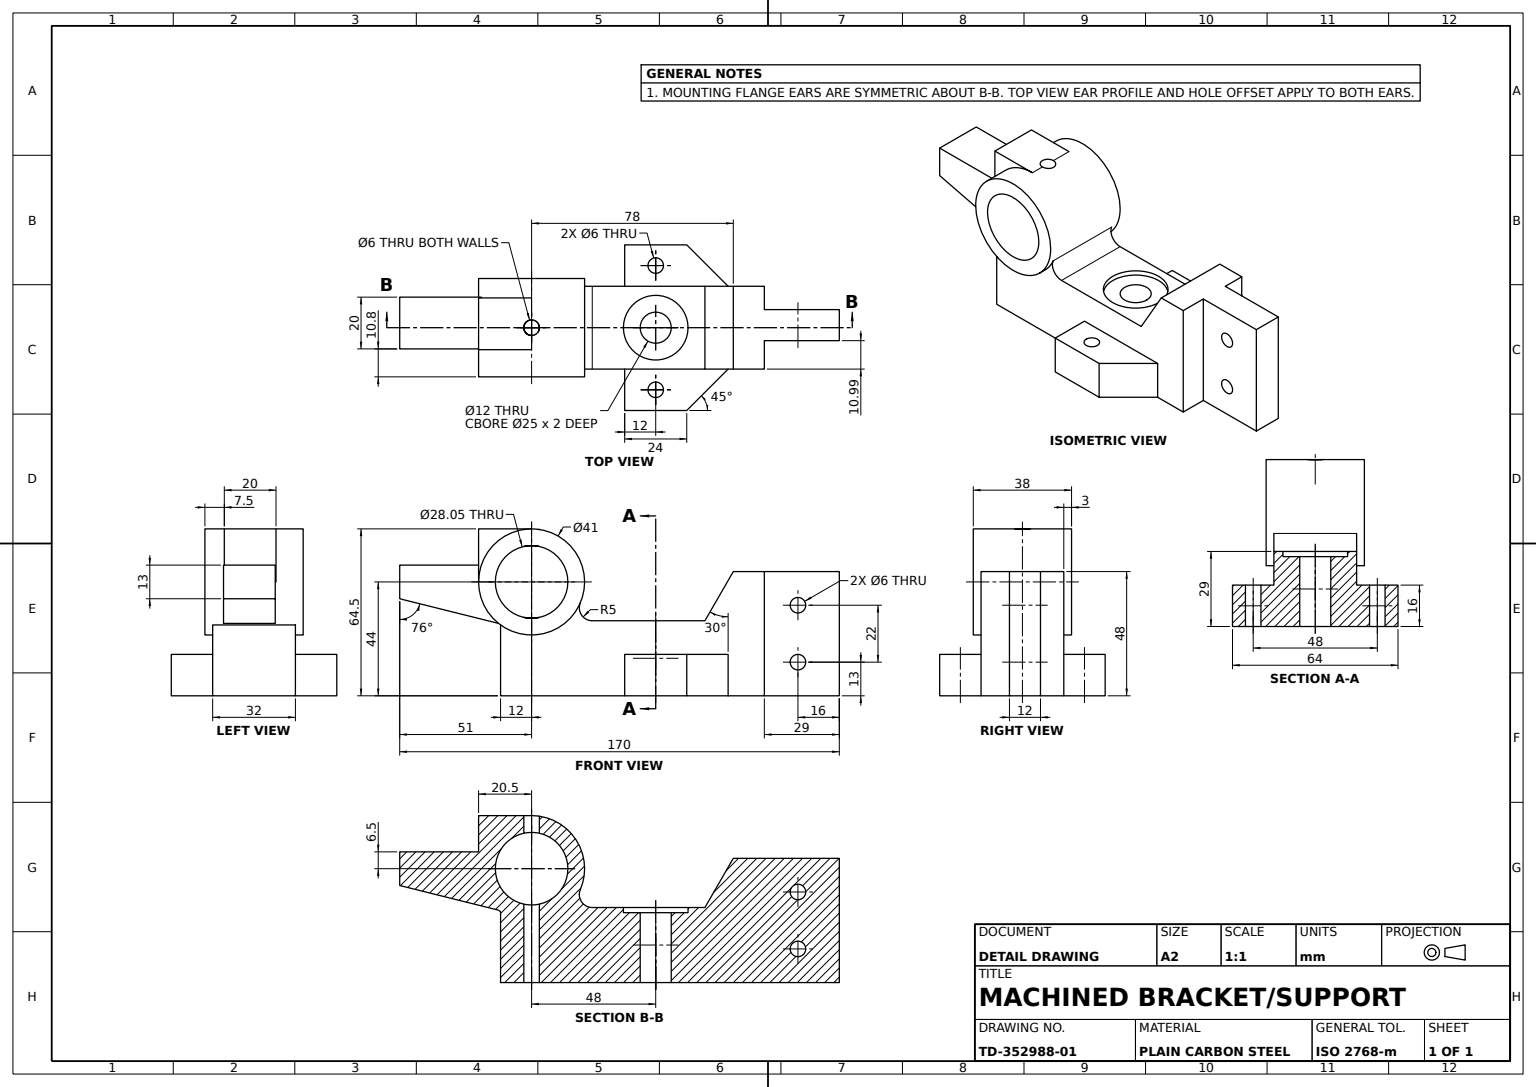
from build123d import *

# Parameters (mm, degrees)
BASE_BLOCK_48MM_DEPTH      = 48
BASE_NOTCH_SKETCH_R        = 3
BASE_NOTCH_CUT_DEPTH       = 67.532624112
ANGLED_ARM_30DEG_DEPTH     = 32
MOUNTING_FLANGE_DEPTH      = 3
MOUNTING_FLANGE_DEPTH_BACK = 35
MOUNTING_FLANGE_SKETCH_R   = 20.5
MOUNTING_FLANGE_SKETCH_R_2 = 14
RAISED_BLOCK_16MM_DEPTH    = 16
POCKET_SKETCH_R            = 3.17708526
POCKET_SKETCH_R_2          = 3.631937334
POCKET_SKETCH_R_3          = 12.5
POCKET_CUT_2MM_DEPTH       = 2
SLOT_SKETCH_R              = 6
SLOT_SKETCH_R_2            = 3
SLOT_CUT_DEPTH             = 112.707383368
CHANNEL_CUT_DEPTH          = 112.05196756
CHANNEL_CUT_DEPTH_BACK     = 112.05196756
CHANNEL_SKETCH_R           = 3
LUG_START                  = -27.5
LUG_A_DEPTH                = 20
LUG_B_DEPTH                = 20
LUG_START_2                = -10.8
LUG_C_DEPTH                = 20
FLANGE_HOLE_DEPTH          = 153.977939634
FLANGE_HOLE_DEPTH_BACK     = 153.977939634
FLANGE_HOLE_SKETCH_R       = 14.02508448
LUG_A_HOLE_DEPTH           = 149.900266997
LUG_A_HOLE_DEPTH_BACK      = 149.900266997
LUG_A_HOLE_SKETCH_R        = 3
ARM_FILLET_R5_R            = 5


with BuildPart() as part:
    # Base Block Sketch → Base Block 48mm (new body)
    with BuildSketch(Plane(origin=(0, 0, 0), x_dir=(1, 0, 0), z_dir=(0, 1, 0))):
        Polygon((12, 0), (41, 0), (41, 12), (12, 12), (12, 21.014044617), (0, 21.014044617), (0, -10.985955383), (12, -10.985955383), align=None)
    extrude(amount=BASE_BLOCK_48MM_DEPTH)

    # Base Notch Sketch → Base Notch Cut (cut, through all)
    with BuildSketch(Plane.XY):
        with Locations((25, 35)):
            Circle(BASE_NOTCH_SKETCH_R)
        with Locations((25, 13)):
            Circle(BASE_NOTCH_SKETCH_R)
    extrude(amount=-BASE_NOTCH_CUT_DEPTH, mode=Mode.SUBTRACT)

    # Angled Arm Sketch → Angled Arm 30deg (add)
    with BuildSketch(Plane.XY.offset(10.985955383)):
        Polygon((0, 48), (-10.969655115, 29), (-90, 29), (-90, 0), (0, 0), align=None)
    extrude(amount=-ANGLED_ARM_30DEG_DEPTH)

    # Mounting Flange Sketch → Mounting Flange (add, two sides: drawn at the far end of the back side and taken through both)
    with BuildSketch(Plane.XY.offset(10.985955383).offset(-MOUNTING_FLANGE_DEPTH_BACK)):
        with Locations((-78, 44)):
            Circle(MOUNTING_FLANGE_SKETCH_R)
        with Locations((-78, 44)):
            Circle(MOUNTING_FLANGE_SKETCH_R_2, mode=Mode.SUBTRACT)
    extrude(amount=MOUNTING_FLANGE_DEPTH + MOUNTING_FLANGE_DEPTH_BACK)

    # Raised Block Sketch → Raised Block 16mm (add)
    with BuildSketch(Plane.XZ):
        Polygon((-42, -37.014044617), (-18, -37.014044617), (-2, -21.014044617), (-42, -21.014044617), align=None)
        Polygon((-42, 10.985955383), (-2, 10.985955383), (-18, 26.985955383), (-42, 26.985955383), align=None)
    extrude(amount=-RAISED_BLOCK_16MM_DEPTH)

    # Pocket Sketch → Pocket Cut 2mm (cut)
    with BuildSketch(Plane(origin=(0, 29, 0), x_dir=(1, 0, 0), z_dir=(0, 1, 0))):
        with Locations((-30, -18.985955383)):
            Circle(POCKET_SKETCH_R)
        with Locations((-30, 29.014044617)):
            Circle(POCKET_SKETCH_R_2)
        with Locations(Location((-30, 5.014044617, 0), (0, 0, 180))):
            Circle(POCKET_SKETCH_R_3)
    extrude(amount=-POCKET_CUT_2MM_DEPTH, mode=Mode.SUBTRACT)

    # Slot Sketch → Slot Cut (cut, through all)
    with BuildSketch(Plane(origin=(0, 27, 0), x_dir=(1, 0, 0), z_dir=(0, 1, 0))):
        with Locations(Location((-30, 5.014044617, 0), (0, 0, 180))):
            Circle(SLOT_SKETCH_R)
        with Locations(Location((-30, -18.985955383, 0), (0, 0, 180))):
            Circle(SLOT_SKETCH_R_2)
        with Locations(Location((-30, 29.014044617, 0), (0, 0, 180))):
            Circle(SLOT_SKETCH_R_2)
    extrude(amount=-SLOT_CUT_DEPTH, mode=Mode.SUBTRACT)

    # Channel Sketch → Channel Cut (cut, two sides: drawn at the far end of the back side and taken through both)
    with BuildSketch(Plane(origin=(0, 29, 0), x_dir=(1, 0, 0), z_dir=(0, 1, 0)).offset(-CHANNEL_CUT_DEPTH_BACK)):
        with Locations(Location((-78, 5.014044617, 0), (0, 0, 180))):
            Circle(CHANNEL_SKETCH_R)
    extrude(amount=CHANNEL_CUT_DEPTH + CHANNEL_CUT_DEPTH_BACK, mode=Mode.SUBTRACT)

    # Lug A Sketch → Lug A (add)
    with BuildSketch(Plane.XY.offset(10.985955383).offset(LUG_START)):
        with BuildLine():
            Line((-90, 64.5), (-78, 64.5))
            ThreePointArc((-78, 64.5), (-84.305720108, 63.50609889), (-90, 60.620770139))
            Line((-90, 60.620770139), (-90, 64.5))
        make_face()
    extrude(amount=LUG_A_DEPTH)

    # Lug B Sketch → Lug B (add)
    with BuildSketch(Plane.XY.offset(10.985955383).offset(LUG_START)):
        with BuildLine():
            Line((-98.5, 44), (-98.5, 64.5))
            Line((-98.5, 64.5), (-90, 64.5))
            Line((-90, 64.5), (-90, 60.620770139))
            ThreePointArc((-90, 60.620770139), (-96.251712248, 53.334077351), (-98.5, 44))
        make_face()
    extrude(amount=LUG_B_DEPTH)

    # Lug C Sketch → Lug C (add)
    with BuildSketch(Plane.XY.offset(13.985955383).offset(LUG_START_2)):
        Polygon((-129, 50.5), (-129, 37.5), (-90, 27.776207889), (-90, 50.5), align=None)
    extrude(amount=-LUG_C_DEPTH)

    # Flange Hole Sketch → Flange Hole (cut, two sides: drawn at the far end of the back side and taken through both)
    with BuildSketch(Plane.XY.offset(13.985955383).offset(-FLANGE_HOLE_DEPTH_BACK)):
        with Locations((-78, 44)):
            Circle(FLANGE_HOLE_SKETCH_R)
    extrude(amount=FLANGE_HOLE_DEPTH + FLANGE_HOLE_DEPTH_BACK, mode=Mode.SUBTRACT)

    # Lug A Hole Sketch → Lug A Hole (cut, two sides: drawn at the far end of the back side and taken through both)
    with BuildSketch(Plane(origin=(0, 64.5, 0), x_dir=(1, 0, 0), z_dir=(0, 1, 0)).offset(-LUG_A_HOLE_DEPTH_BACK)):
        with Locations(Location((-78, 5.014044617, 0), (0, 0, 180))):
            Circle(LUG_A_HOLE_SKETCH_R)
    extrude(amount=LUG_A_HOLE_DEPTH + LUG_A_HOLE_DEPTH_BACK, mode=Mode.SUBTRACT)

    # Arm Fillet R5
    arm_fillet_r5_edges = [part.edges().sort_by_distance(p)[0] for p in [
        (-64.026811388, 29, -5.014044617),
    ]]
    fillet(arm_fillet_r5_edges, radius=ARM_FILLET_R5_R)


solid = part.part
